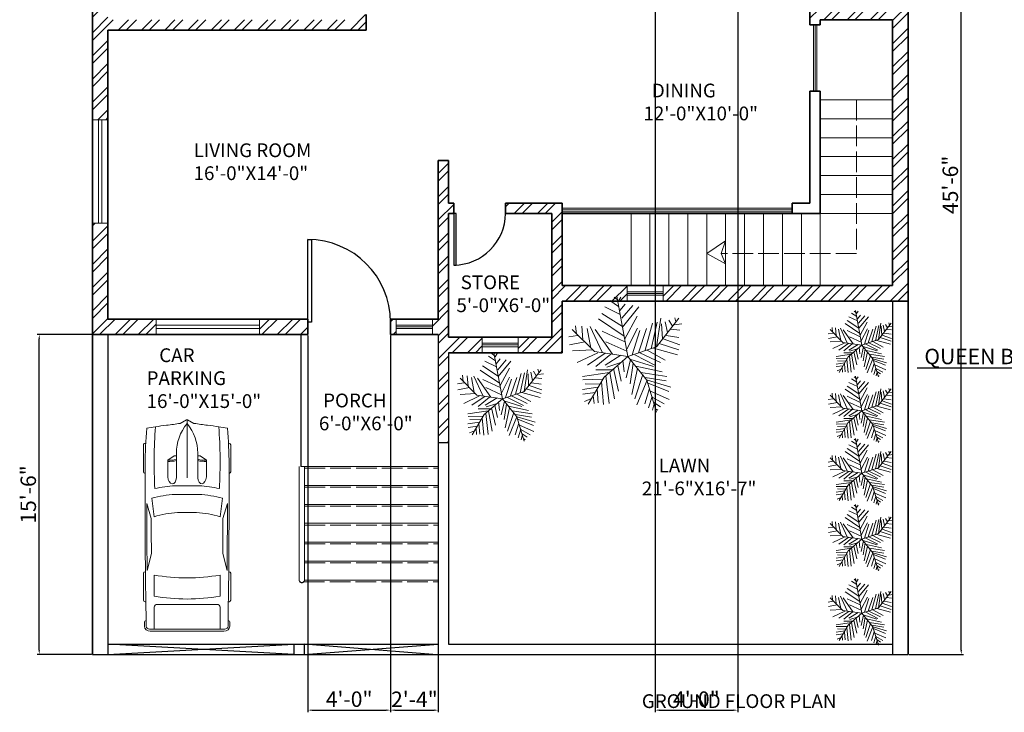
# Model space of a CAD drawing. Units: inches. Extents: x 600 to 1805, y 898 to 2057.
# Tile 2 of 5: x 600 to 1172, y 1419 to 1822. Entities that reach past the tile are written whole.
import ezdxf

# ---------------------------------------------------------------- set-up
doc = ezdxf.new("R2010")
doc.units = ezdxf.units.IN
doc.linetypes.add('ACAD_ISO02W100', pattern=[15, 12, -3])
for name, color, linetype, lineweight in [('A-ANNO-DIMS', 2, 'Continuous', 18), ('A-ANNO-PATH', 2, 'ACAD_ISO02W100', 13), ('A-ANNO-SYMB', 2, 'Continuous', 13), ('A-ANNO-TEXT', 7, 'Continuous', 25), ('A-AREA-IDEN', 7, 'Continuous', 18), ('A-DOOR', 4, 'Continuous', 25), ('A-FLOR', 7, 'Continuous', 25), ('A-FLOR-STRS', 3, 'Continuous', 20), ('A-FLOR-STRS-HIDN', 3, 'ACAD_ISO02W100', 13), ('A-WALL', 7, 'Continuous', 35), ('A-WALL-PATT', 252, 'Continuous', 13), ('C-PRKG-VEH', 8, 'Continuous', 13), ('C-SITE', 7, 'Continuous', 25), ('L-PLNT', 94, 'Continuous', 13)]:
    doc.layers.add(name, color=color, linetype=linetype, lineweight=lineweight)
doc.layers.add('A-GLAZ', color=244, linetype='Continuous', lineweight=20, true_color=0x991b1e)
doc.styles.get("Standard").update_dxf_attribs({"font": 'arial.ttf'})
doc.dimstyles.new('ISO-25', dxfattribs={"dimtxt": 9, "dimasz": 2.5, "dimexe": 1.25, "dimexo": 0.625, "dimtad": 1, "dimlunit": 3, "dimtxsty": 'Standard', "dimcen": 2.5, "dimadec": 0, "dimazin": 0, "dimtfac": 1, "dimtmove": 0, "dimatfit": 3, "dimfxl": 1, "dimarcsym": 0})

# ---------------------------------------------------------------- blocks, each defined once
blk = doc.blocks.new('*U5')
for p, q in [((0, 0), (0, 6)), ((40, 0), (40, 6))]:
    blk.add_line(p, q)
blk.add_lwpolyline([(0, 0), (0, -40), (1.75, -40), (1.75, 0)], close=True)
blk.add_arc((0, 0), 40, 270, 0)
blk = doc.blocks.new('*U2')
for p, q in [((0, 0), (0, -6)), ((40, 0), (40, -6))]:
    blk.add_line(p, q)
blk.add_lwpolyline([(0, 0), (0, 40), (1.75, 40), (1.75, 0)], close=True)
blk.add_arc((0, 0), 40, 0, 90)
blk = doc.blocks.new('*U7')
for p, q in [((21.1, 37.41), (21.1, 36.83)), ((46.55, 38.89), (22.35, 38.89)), ((47.8, 37.39), (47.8, 37.41)), ((87.99, 31.87), (74.76, 35.92)), ((134.31, 35.6), (119.29, 31.78)), ((135.45, 37.07), (135.45, 37.41)), ((136.7, 38.89), (160.9, 38.89)), ((162.15, 37.41), (162.15, 36.77)), ((70.03, 31.54), (86.41, 29.35)), ((138.42, 29.35), (157.25, 29.35)), ((164.52, 26.39), (164.52, -26.39)), ((186.47, 29.35), (167.01, 29.35)), ((186.47, -33.5), (186.47, 33.5)), ((188.4, -32.76), (188.4, 32.76)), ((29.77, 9.51), (51.68, 9.51)), ((32.12, 9.51), (32.12, 11.15)), ((32.27, 11.63), (36.13, 17.17)), ((36.13, 17.17), (50.94, 17.17)), ((58.92, -10.77), (58.92, 10.77)), ((66.55, -10.53), (66.55, 10.53)), ((186.47, -10.53), (186.47, 10.53)), ((3.27, 6.13), (0.1, 0.41)), ((82.74, 8.5), (82.74, -8.5)), ((0, 0), (51.68, 0)), ((0.1, -0.41), (3.27, -6.13)), ((29.77, -9.51), (51.68, -9.51)), ((32.12, -9.51), (32.12, -11.15)), ((32.27, -11.63), (36.13, -17.17)), ((36.13, -17.17), (50.94, -17.17)), ((86.41, -29.35), (70.03, -31.54)), ((87.99, -31.87), (74.76, -35.92)), ((134.31, -35.6), (119.29, -31.78)), ((157.25, -29.35), (138.42, -29.35)), ((167.01, -29.35), (186.47, -29.35)), ((21.1, -37.41), (21.1, -36.83)), ((46.55, -38.89), (22.35, -38.89)), ((47.8, -37.39), (47.8, -37.41)), ((135.45, -37.07), (135.45, -37.41)), ((136.7, -38.89), (160.9, -38.89)), ((162.15, -37.41), (162.15, -36.77))]:
    blk.add_line(p, q)
for centre, major_axis, ratio, start_param, end_param in [((266.03, -27.52), (0, 313.31), 0.842304, 1.367076, 1.39176), ((41.19, -490.86), (0, 528.23), 0.842304, 0.00281, 0.075598), ((22.35, 37.41), (0, -1.48), 0.842304, 3.141593, 4.712389), ((64.48, -10555.62), (0, 10593.03), 0.842304, -0.013397, 0.002797), ((46.55, 37.41), (0, 1.48), 0.842304, -1.570796, 0), ((64.48, -10555.62), (0, -10591.55), 0.842304, 3.133765, 3.140441), ((136.7, 37.41), (0, -1.48), 0.842304, 3.141593, 4.712389), ((160.9, 37.41), (0, 1.48), 0.842304, -1.570796, 0), ((180.63, 35.84), (0, 2.22), 0.842304, -0.013017, 1.249894), ((64.48, -10556.36), (0, 10595.31), 0.842304, -0.013397, -0.013017), ((183.98, 33.5), (0, -2.96), 0.842304, 1.570796, 3.128196), ((183.98, 32.76), (0, -5.25), 0.842304, 1.570796, 3.128196), ((259.18, -27.52), (0, -305.3), 0.842304, 4.528606, 4.561838), ((37.47, -593.96), (0, -623.33), 0.842304, 3.096046, 3.200911), ((134.4, 5.39), (0, -89.78), 0.842304, 4.449482, 4.652344), ((135.29, 5.39), (0, 81.77), 0.842304, 1.245306, 1.50788), ((149.6, 2.8), (0, -79.58), 0.842304, 4.372215, 4.640744), ((95.79, -3666.35), (0, -3698.24), 0.842304, 3.134049, 3.144098), ((17.08, 0), (0, 147.02), 0.842304, 4.511394, 4.913384), ((35.91, 0), (0, 147.02), 0.842304, 4.511394, 4.913384), ((167.01, 26.39), (0, 2.96), 0.842304, 0, 1.570796), ((-204.49, 52.4), (0, -250.96), 0.842304, 1.385369, 1.434372), ((29.77, -46.66), (0, 56.17), 0.842304, 0, 0.590319), ((32.75, 11.15), (0, 0.74), 0.842304, 0.879714, 1.570796), ((13.04, 17.01), (0, 27.42), 0.842304, 4.435146, 4.718221), ((14.2, 17.01), (0, 27.42), 0.842304, 4.435146, 4.718221), ((50.79, 13.34), (6.34, -0.36), 0.603834, -1.395552, 1.581315), ((0.62, 0), (0, -0.74), 0.842304, 4.131459, 5.293319), ((-204.49, -52.4), (0, 250.96), 0.842304, -1.434372, -1.385369), ((29.77, 46.66), (0, 56.17), 0.842304, 2.551274, 3.141593), ((149.6, -2.8), (0, -79.58), 0.842304, -1.499151, -1.230623), ((32.75, -11.15), (0, -0.74), 0.842304, 4.712389, 5.403472), ((13.04, -17.01), (0, -27.42), 0.842304, 1.564964, 1.848039), ((14.2, -17.01), (0, -27.42), 0.842304, 1.564964, 1.848039), ((134.4, -5.39), (0, -89.78), 0.842304, -1.510751, -1.307889), ((135.29, -5.39), (0, -81.77), 0.842304, -1.50788, -1.245306), ((259.18, 27.52), (0, 305.3), 0.842304, 1.721348, 1.754579), ((266.03, 27.52), (0, 313.31), 0.842304, 1.749832, 1.774517), ((37.47, 593.96), (0, -623.33), 0.842304, -0.059319, 0.045547), ((95.79, 3666.35), (0, -3698.24), 0.842304, -0.002505, 0.007544), ((167.01, -26.39), (0, -2.96), 0.842304, 4.712389, 6.283185), ((183.98, -33.5), (0, 2.96), 0.842304, 3.15499, 4.712389), ((183.98, -32.76), (0, -5.25), 0.842304, 0.013397, 1.570796), ((41.19, 490.86), (0, -528.23), 0.842304, -0.075598, -0.00281), ((22.35, -37.41), (0, 1.48), 0.842304, 1.570796, 3.141593), ((64.48, 10555.62), (0, 10593.03), 0.842304, 3.138796, 3.15499), ((46.55, -37.41), (0, -1.48), 0.842304, 0, 1.570796), ((64.48, 10555.62), (0, -10591.55), 0.842304, 0.001152, 0.007828), ((136.7, -37.41), (0, -1.48), 0.842304, -1.570796, 0), ((160.9, -37.41), (0, 1.48), 0.842304, 3.141593, 4.712389), ((180.63, -35.84), (0, -2.22), 0.842304, -1.249894, 0.013017), ((64.48, 10556.36), (0, 10595.31), 0.842304, 3.15461, 3.15499)]:
    blk.add_ellipse(centre, major_axis=major_axis, ratio=ratio, start_param=start_param, end_param=end_param)
at = {"extrusion": (0, 0, -1)}
blk.add_ellipse((50.79, -13.34), major_axis=(6.34, 0.36), ratio=0.603834, start_param=-1.395552, end_param=1.581315, dxfattribs=at)
blk = doc.blocks.new('*U12')
for p, q in [((-10.186, 53.64), (-13.084, 55.962)), ((0, 0), (-10.5, 57)), ((-9.099, 51.782), (-6.563, 55.962)), ((-7.288, 39.707), (-21.778, 46.673)), ((-8.737, 47.138), (-17.069, 52.711)), ((-7.65, 43.423), (-2.578, 49.46)), ((-5.839, 35.992), (4.667, 48.067)), ((-5.114, 27.632), (10.463, 46.673)), ((-5.114, 28.097), (-24.676, 40.636)), ((-2.941, 16.486), (8.652, 37.85)), ((-48.585, 21.131), (-49.309, 29.026)), ((-43.513, 28.561), (-42.427, 15.558)), ((-35.544, 28.097), (-24.314, 3.947)), ((-3.665, 19.273), (-27.574, 35.527)), ((16.259, 5.805), (23.142, 31.348)), ((22.055, 7.198), (27.489, 32.277)), ((27, 9), (48, 36)), ((27.127, 9.056), (31.112, 35.992)), ((31.836, 30.883), (32.561, 16.486)), ((35.096, 32.741), (37.27, 22.524)), ((38.719, 34.134), (41.979, 28.561)), ((43.791, 29.954), (51.036, 30.883)), ((44.153, 36.456), (45.239, 32.741)), ((-47.498, 19.737), (-55.83, 18.344)), ((-31.5, 4.5), (-52.5, 25.5)), ((-38.442, 26.239), (-34.819, 7.663)), ((-14.533, 2.09), (-30.834, 25.31)), ((-24.314, 23.917), (-2.941, 13.7)), ((-1.129, 6.734), (9.014, 26.704)), ((3.942, 1.625), (11.187, 24.381)), ((10.101, 3.483), (17.708, 26.239)), ((36.183, 19.737), (48.137, 17.88)), ((40.53, 25.775), (48.862, 24.846)), ((-40.615, 13.7), (-55.105, 10.913)), ((-20.691, 13.7), (-1.129, 4.876)), ((29.662, 12.307), (48.137, 6.269)), ((33.285, 16.486), (48.862, 10.913)), ((-33.37, 6.269), (-52.207, 5.34)), ((-28.299, 3.483), (-47.86, -5.805)), ((-21.416, 3.018), (-38.079, -8.128)), ((0, 0), (-31.5, 4.5)), ((-15.982, 2.09), (-30.11, -9.521)), ((0, 0), (-22.5, -19.5)), ((-6.563, 1.161), (-21.416, -8.128)), ((0, 0), (27, 9)), ((0, 0), (18, -22.5)), ((6.478, 1.625), (26.04, -8.592)), ((11.187, 3.483), (30.749, -5.805)), ((18.07, 5.805), (35.096, -3.483)), ((24.229, 7.663), (46.688, 1.625)), ((-6.563, -5.805), (-19.967, -9.985)), ((-9.461, -8.592), (-6.201, -23.453)), ((-4.752, -3.483), (-3.665, -14.629)), ((2.493, -3.019), (-1.491, -20.202)), ((1.769, -2.555), (24.229, -9.521)), ((5.029, -6.27), (2.131, -25.775)), ((7.565, -9.056), (32.198, -14.629)), ((-17.431, -15.094), (-42.789, -18.809)), ((-15.257, -12.772), (-30.11, -12.772)), ((-20.691, -18.345), (-17.793, -44.352)), ((-17.069, -15.094), (-12.721, -40.172)), ((-13.446, -11.378), (-8.737, -32.741)), ((9.014, -11.378), (3.58, -35.992)), ((14.085, -16.951), (6.478, -40.172)), ((12.274, -15.094), (36.907, -18.809)), ((-24.314, -21.596), (-42.427, -22.06)), ((-26.849, -26.24), (-40.253, -25.775)), ((-22.5, -19.5), (-37.5, -45)), ((-25.038, -23.918), (-22.865, -45.281)), ((18.07, -22.524), (8.289, -45.745)), ((16.259, -19.738), (36.183, -22.989)), ((18, -22.5), (27, -52.5)), ((18.433, -22.524), (40.53, -29.026)), ((19.157, -25.311), (38.719, -33.206)), ((-28.299, -29.026), (-42.789, -31.348)), ((-30.834, -34.135), (-42.427, -35.528)), ((-32.646, -36.921), (-31.921, -44.352)), ((-29.023, -30.884), (-27.936, -43.887)), ((20.244, -30.419), (15.897, -44.816)), ((21.331, -32.741), (39.081, -40.636)), ((-34.457, -39.708), (-40.978, -42.494)), ((22.78, -37.85), (19.519, -48.532)), ((22.78, -38.314), (34.372, -44.816)), ((24.591, -45.745), (23.142, -50.854)), ((24.591, -43.423), (30.749, -47.603)), ((26.764, -49.925), (28.213, -50.854))]:
    blk.add_line(p, q)
blk = doc.blocks.new('WIN-60x9')
for p, q in [((60, 5.5), (0, 5.5)), ((60, 3.5), (0, 3.5))]:
    blk.add_line(p, q)
blk.add_lwpolyline([(60, 0), (60, 9), (0, 9), (0, 0)], close=True)
blk = doc.blocks.new('VENT-21x9')
for p, q in [((0, 5.5), (21, 5.5)), ((0, 4.5), (21, 4.5)), ((0, 3.5), (21, 3.5))]:
    blk.add_line(p, q)
blk.add_lwpolyline([(21, 9), (21, 0), (0, 0), (0, 9)], close=True)
blk = doc.blocks.new('*D26')
at = {"layer": 'A-ANNO-DIMS', "color": 0, "lineweight": -2, "transparency": 16777216}
for p, q in [((1257.94, 1608), (1257.94, 1620.63)), ((1337.94, 1608), (1337.94, 1620.63)), ((1257.94, 1619.38), (1121.8, 1619.38)), ((1335.44, 1619.38), (1260.44, 1619.38))]:
    blk.add_line(p, q, dxfattribs=at)
at = {"layer": 'A-ANNO-DIMS', "color": 0, "transparency": 16777216}
for points in [[(1260.44, 1619.79), (1260.44, 1618.96), (1257.94, 1619.38)], [(1335.44, 1619.79), (1335.44, 1618.96), (1337.94, 1619.38)]]:
    blk.add_solid(points, dxfattribs=at)
at = {"layer": 'Defpoints', "color": 0, "transparency": 16777216}
for p in [(1257.94, 1619.38), (1257.94, 1607.38), (1337.94, 1607.38)]:
    blk.add_point(p, dxfattribs=at)
at = {"layer": 'A-ANNO-DIMS', "color": 0, "transparency": 16777216, "insert": (1188.62, 1624.93), "char_height": 9, "attachment_point": 5}
blk.add_mtext('QUEEN BED 6\'-8" TYP.', dxfattribs=at)
blk = doc.blocks.new('*D32')
at = {"layer": 'A-ANNO-DIMS', "color": 0, "lineweight": -2, "transparency": 16777216}
for p, q in [((1117.01, 1998.86), (1148.59, 1998.86)), ((1147.34, 1455.36), (1147.34, 1996.36)), ((1117.01, 1452.86), (1148.59, 1452.86))]:
    blk.add_line(p, q, dxfattribs=at)
at = {"layer": 'A-ANNO-DIMS', "color": 0, "transparency": 16777216}
for points in [[(1146.92, 1996.36), (1147.75, 1996.36), (1147.34, 1998.86)], [(1146.92, 1455.36), (1147.75, 1455.36), (1147.34, 1452.86)]]:
    blk.add_solid(points, dxfattribs=at)
at = {"layer": 'Defpoints', "color": 0, "transparency": 16777216}
for p in [(1116.39, 1998.86), (1147.34, 1998.86), (1116.39, 1452.86)]:
    blk.add_point(p, dxfattribs=at)
at = {"layer": 'A-ANNO-DIMS', "color": 0, "transparency": 16777216, "insert": (1142.12, 1725.86), "char_height": 9, "attachment_point": 5, "rotation": 90}
blk.add_mtext('45\'-6"', dxfattribs=at)
blk = doc.blocks.new('*D33')
at = {"layer": 'A-ANNO-DIMS', "color": 0, "lineweight": -2, "transparency": 16777216}
for p, q in [((641.76, 1638.86), (610.19, 1638.86)), ((611.44, 1455.36), (611.44, 1636.36)), ((641.76, 1452.86), (610.19, 1452.86))]:
    blk.add_line(p, q, dxfattribs=at)
at = {"layer": 'A-ANNO-DIMS', "color": 0, "transparency": 16777216}
for points in [[(611.02, 1636.36), (611.85, 1636.36), (611.44, 1638.86)], [(611.02, 1455.36), (611.85, 1455.36), (611.44, 1452.86)]]:
    blk.add_solid(points, dxfattribs=at)
at = {"layer": 'Defpoints', "color": 0, "transparency": 16777216}
for p in [(611.44, 1638.86), (642.39, 1638.86), (642.39, 1452.86)]:
    blk.add_point(p, dxfattribs=at)
at = {"layer": 'A-ANNO-DIMS', "color": 0, "transparency": 16777216, "insert": (606.22, 1545.86), "char_height": 9, "attachment_point": 5, "rotation": 90}
blk.add_mtext('15\'-6"', dxfattribs=at)
blk = doc.blocks.new('*D34')
at = {"layer": 'A-ANNO-DIMS', "color": 0, "lineweight": -2, "transparency": 16777216}
for p, q in [((815.57, 1638.23), (815.57, 1419.24)), ((843.39, 1638.23), (843.39, 1419.24)), ((818.07, 1420.49), (840.89, 1420.49))]:
    blk.add_line(p, q, dxfattribs=at)
at = {"layer": 'A-ANNO-DIMS', "color": 0, "transparency": 16777216}
for points in [[(818.07, 1420.9), (818.07, 1420.07), (815.57, 1420.49)], [(840.89, 1420.9), (840.89, 1420.07), (843.39, 1420.49)]]:
    blk.add_solid(points, dxfattribs=at)
at = {"layer": 'Defpoints', "color": 0, "transparency": 16777216}
for p in [(815.57, 1638.86), (843.39, 1638.86), (843.39, 1420.49)]:
    blk.add_point(p, dxfattribs=at)
at = {"layer": 'A-ANNO-DIMS', "color": 0, "transparency": 16777216, "insert": (829.48, 1425.63), "char_height": 9, "attachment_point": 5}
blk.add_mtext('2\'-4"', dxfattribs=at)
blk = doc.blocks.new('*D35')
at = {"layer": 'A-ANNO-DIMS', "color": 0, "lineweight": -2, "transparency": 16777216}
for p, q in [((767.57, 1638.23), (767.57, 1419.24)), ((815.57, 1638.23), (815.57, 1419.24)), ((770.07, 1420.49), (813.07, 1420.49))]:
    blk.add_line(p, q, dxfattribs=at)
at = {"layer": 'A-ANNO-DIMS', "color": 0, "transparency": 16777216}
for points in [[(770.07, 1420.9), (770.07, 1420.07), (767.57, 1420.49)], [(813.07, 1420.9), (813.07, 1420.07), (815.57, 1420.49)]]:
    blk.add_solid(points, dxfattribs=at)
at = {"layer": 'Defpoints', "color": 0, "transparency": 16777216}
for p in [(767.57, 1638.86), (815.57, 1638.86), (815.57, 1420.49)]:
    blk.add_point(p, dxfattribs=at)
at = {"layer": 'A-ANNO-DIMS', "color": 0, "transparency": 16777216, "insert": (791.57, 1425.71), "char_height": 9, "attachment_point": 5}
blk.add_mtext('4\'-0"', dxfattribs=at)
blk = doc.blocks.new('*D57')
at = {"layer": 'A-ANNO-DIMS', "color": 0, "lineweight": -2, "transparency": 16777216}
for p, q in [((969.39, 1863.23), (969.39, 1419.24)), ((1017.39, 1863.23), (1017.39, 1419.24)), ((971.89, 1420.49), (1014.89, 1420.49))]:
    blk.add_line(p, q, dxfattribs=at)
at = {"layer": 'A-ANNO-DIMS', "color": 0, "transparency": 16777216}
for points in [[(971.89, 1420.9), (971.89, 1420.07), (969.39, 1420.49)], [(1014.89, 1420.9), (1014.89, 1420.07), (1017.39, 1420.49)]]:
    blk.add_solid(points, dxfattribs=at)
at = {"layer": 'Defpoints', "color": 0, "transparency": 16777216}
for p in [(969.39, 1863.86), (1017.39, 1863.86), (1017.39, 1420.49)]:
    blk.add_point(p, dxfattribs=at)
at = {"layer": 'A-ANNO-DIMS', "color": 0, "transparency": 16777216, "insert": (993.39, 1425.71), "char_height": 9, "attachment_point": 5}
blk.add_mtext('4\'-0"', dxfattribs=at)

msp = doc.modelspace()

# ---------------------------------------------------------------- hatches: boundary and pattern name
at = {"layer": 'A-WALL-PATT'}
h = msp.add_hatch(dxfattribs=at)
h.set_pattern_fill('ANSI32', color=256)
h.paths.add_polyline_path([(651.387, 1875.859), (642.387, 1875.859), (642.387, 1763.631), (651.387, 1763.631), (651.387, 1815.859), (801.387, 1815.859), (801.387, 1824.859), (795.987, 1824.859), (795.387, 1824.859), (795.387, 1821.859), (651.387, 1821.859)])
h.paths.add_polyline_path([(795.387, 1989.859), (795.387, 1860.859), (801.387, 1860.859), (801.387, 1887.859), (804.387, 1887.859), (804.387, 1892.359), (804.387, 1893.859), (801.387, 1893.859), (801.387, 1989.859), (807.224, 1989.859), (807.224, 1998.859), (753.387, 1998.859), (753.387, 1989.859)])
h.paths.add_polyline_path([(693.387, 1989.859), (693.387, 1998.859), (642.387, 1998.859), (642.387, 1935.859), (651.387, 1935.859), (651.387, 1989.859)])
h.paths.add_polyline_path([(828.224, 1998.859), (828.224, 1989.859), (861.387, 1989.859), (861.387, 1893.859), (834.387, 1893.859), (834.387, 1887.859), (861.387, 1887.859), (894.387, 1887.859), (894.387, 1892.359), (894.387, 1893.859), (867.387, 1893.859), (867.387, 1989.859), (894.316, 1989.859), (894.316, 1998.859)])
h = msp.add_hatch(dxfattribs=at)
h.set_pattern_fill('ANSI32', color=256)
h.paths.add_polyline_path([(933.387, 1989.859), (963.387, 1989.859), (963.387, 1998.859), (915.316, 1998.859), (915.316, 1989.859), (927.387, 1989.859), (927.387, 1893.859), (924.387, 1893.859), (924.387, 1892.359), (924.387, 1887.859), (927.387, 1887.859), (927.387, 1863.859), (969.387, 1863.859), (969.387, 1869.859), (933.387, 1869.859)])
h.paths.add_polyline_path([(1059.387, 1998.859), (1023.387, 1998.859), (1023.387, 1989.859), (1053.387, 1989.859), (1053.387, 1869.859), (1017.387, 1869.859), (1017.387, 1863.859), (1062.387, 1863.859), (1062.387, 1867.459), (1062.387, 1869.859), (1059.387, 1869.859)], flags=17)
h.paths.add_polyline_path([(1116.387, 1998.859), (1107.387, 1998.859), (1107.387, 1869.859), (1086.387, 1869.859), (1086.387, 1863.859), (1107.387, 1863.859), (1107.387, 1827.859), (1059.387, 1827.859), (1059.387, 1818.859), (1065.387, 1818.859), (1065.387, 1821.859), (1107.387, 1821.859), (1107.387, 1667.256), (974.103, 1667.256), (974.103, 1658.256), (1116.387, 1658.256)])
h.paths.add_polyline_path([(953.103, 1667.256), (915.387, 1667.256), (915.387, 1715.256), (882.387, 1715.256), (882.387, 1709.256), (909.387, 1709.256), (909.387, 1637.256), (889.887, 1637.256), (889.887, 1628.256), (915.387, 1628.256), (915.387, 1658.256), (953.103, 1658.256)])
h.paths.add_polyline_path([(868.887, 1637.256), (849.387, 1637.256), (849.387, 1709.256), (852.387, 1709.256), (852.387, 1713.756), (852.387, 1715.256), (849.387, 1715.256), (849.387, 1740.017), (843.387, 1740.017), (843.387, 1647.859), (839.976, 1647.859), (839.976, 1638.859), (843.387, 1638.859), (843.387, 1576.163), (849.387, 1576.163), (849.387, 1628.256), (868.887, 1628.256)])
h.paths.add_polyline_path([(767.566, 1646.059), (767.566, 1647.859), (739.476, 1647.859), (739.476, 1638.859), (767.566, 1638.859)])
h = msp.add_hatch(dxfattribs=at)
h.set_pattern_fill('ANSI32', color=256)
h.paths.add_polyline_path([(679.476, 1647.859), (651.387, 1647.859), (651.387, 1703.631), (642.387, 1703.631), (642.387, 1638.859), (679.476, 1638.859)])
h.paths.add_polyline_path([(818.976, 1647.859), (815.566, 1647.859), (815.566, 1638.859), (818.976, 1638.859)])

# ---------------------------------------------------------------- linework, layer by layer
at = {"layer": 'A-ANNO-PATH'}
for p, q in [((1086.387, 1775.256), (1086.387, 1685.977)), ((1086.387, 1685.977), (1007.718, 1685.977))]:
    msp.add_line(p, q, dxfattribs=at)
at = {"layer": 'A-ANNO-SYMB'}
for p, q in [((999.387, 1685.977), (1010.387, 1693.236)), ((1010.387, 1693.236), (1007.718, 1685.977)), ((1010.387, 1679.972), (999.387, 1685.977)), ((1007.718, 1685.977), (1010.387, 1679.972))]:
    msp.add_line(p, q, dxfattribs=at)
at = {"layer": 'A-DOOR'}
for p, q in [((651.387, 1452.859), (759.445, 1458.859)), ((759.445, 1452.859), (651.387, 1458.859)), ((759.445, 1458.859), (759.445, 1452.859)), ((765.445, 1458.859), (765.445, 1452.859)), ((765.445, 1452.859), (843.387, 1458.859)), ((840.239, 1452.859), (765.445, 1458.859))]:
    msp.add_line(p, q, dxfattribs=at)
at = {"layer": 'A-FLOR'}
msp.add_line((763.566, 1638.859), (763.566, 1562.113), dxfattribs=at)
at = {"layer": 'A-FLOR-STRS'}
for p, q in [((1065.387, 1775.256), (1107.387, 1775.256)), ((1065.387, 1764.256), (1107.387, 1764.256)), ((1065.387, 1753.256), (1107.387, 1753.256)), ((1065.387, 1742.256), (1107.387, 1742.256)), ((1065.387, 1731.256), (1107.387, 1731.256)), ((1065.387, 1720.256), (1107.387, 1720.256)), ((955.387, 1709.256), (955.387, 1667.256)), ((966.387, 1709.256), (966.387, 1667.256)), ((977.387, 1709.256), (977.387, 1667.256)), ((988.387, 1709.256), (988.387, 1667.256)), ((999.387, 1709.256), (999.387, 1667.256)), ((1010.387, 1709.256), (1010.387, 1667.256)), ((1021.387, 1709.256), (1021.387, 1667.256)), ((1032.387, 1709.256), (1032.387, 1667.256)), ((1043.387, 1709.256), (1043.387, 1667.256)), ((1054.387, 1709.256), (1054.387, 1667.256)), ((1065.387, 1709.256), (1065.387, 1667.256)), ((1065.387, 1709.256), (1107.387, 1709.256)), ((762.566, 1562.113), (762.566, 1496.113)), ((763.566, 1562.113), (843.387, 1562.113)), ((765.566, 1562.113), (765.566, 1496.113)), ((765.566, 1551.113), (843.387, 1551.113)), ((765.566, 1540.113), (843.387, 1540.113)), ((765.566, 1529.113), (843.387, 1529.113)), ((765.566, 1518.113), (843.387, 1518.113)), ((765.566, 1507.113), (843.387, 1507.113)), ((765.566, 1496.113), (843.387, 1496.113))]:
    msp.add_line(p, q, dxfattribs=at)
for centre, radius, start, end in [((764.066, 1495.962), 1.508, 174.26491, 5.73509), ((764.066, 1496.149), 1.501, 182.13798, 357.86202)]:
    msp.add_arc(centre, radius, start, end, dxfattribs=at)
at = {"layer": 'A-FLOR-STRS-HIDN'}
for p, q in [((765.566, 1561.113), (843.387, 1561.113)), ((765.566, 1550.113), (843.387, 1550.113)), ((765.566, 1539.113), (843.387, 1539.113)), ((765.566, 1528.113), (843.387, 1528.113)), ((765.566, 1517.113), (843.387, 1517.113)), ((765.566, 1506.113), (843.387, 1506.113)), ((765.311, 1495.113), (843.387, 1495.113))]:
    msp.add_line(p, q, dxfattribs=at)
at = {"layer": 'A-GLAZ'}
for p, q in [((1061.387, 1818.859), (1061.387, 1780.295)), ((1062.387, 1818.859), (1062.387, 1780.295)), ((1063.387, 1818.859), (1063.387, 1780.295)), ((1048.968, 1712.256), (915.387, 1712.256)), ((1048.968, 1711.256), (915.387, 1711.256)), ((1048.968, 1710.256), (915.387, 1710.256))]:
    msp.add_line(p, q, dxfattribs=at)
at = {"layer": 'A-WALL'}
for p, q in [((642.387, 1998.859), (642.387, 1452.859)), ((1116.387, 1998.859), (1116.387, 1452.859)), ((1059.387, 1827.859), (1059.387, 1818.859)), ((801.387, 1824.859), (801.387, 1815.859)), ((1065.387, 1821.859), (1107.387, 1821.859)), ((1065.387, 1821.859), (1065.387, 1818.859)), ((1107.387, 1821.859), (1107.387, 1667.256)), ((651.387, 1815.859), (801.387, 1815.859)), ((651.387, 1815.859), (651.387, 1647.859)), ((1065.387, 1818.859), (1059.387, 1818.859)), ((1059.387, 1780.295), (1059.387, 1715.256)), ((1065.387, 1780.295), (1059.387, 1780.295)), ((1065.387, 1780.295), (1065.387, 1709.256)), ((843.387, 1740.017), (843.387, 1647.859)), ((843.387, 1740.017), (849.387, 1740.017)), ((849.387, 1740.017), (849.387, 1715.256)), ((849.387, 1715.256), (852.387, 1715.256)), ((852.387, 1715.256), (852.387, 1709.256)), ((882.387, 1715.256), (882.387, 1709.256)), ((882.387, 1715.256), (915.387, 1715.256)), ((915.387, 1715.256), (915.387, 1667.256)), ((1048.968, 1709.256), (1048.968, 1715.256)), ((1048.968, 1715.256), (1059.387, 1715.256)), ((849.387, 1709.256), (852.387, 1709.256)), ((849.387, 1709.256), (849.387, 1637.256)), ((882.387, 1709.256), (909.387, 1709.256)), ((909.387, 1709.256), (909.387, 1637.256)), ((915.387, 1709.256), (1065.387, 1709.256)), ((915.387, 1667.256), (1107.387, 1667.256)), ((915.387, 1658.256), (1116.387, 1658.256)), ((915.387, 1658.256), (915.387, 1628.256)), ((651.387, 1647.859), (767.566, 1647.859)), ((767.566, 1638.859), (767.566, 1647.859)), ((815.566, 1638.859), (815.566, 1647.859)), ((815.566, 1647.859), (843.387, 1647.859)), ((642.387, 1638.859), (767.566, 1638.859)), ((815.566, 1638.859), (843.387, 1638.859)), ((849.387, 1637.256), (909.387, 1637.256)), ((849.387, 1628.256), (915.387, 1628.256))]:
    msp.add_line(p, q, dxfattribs=at)
at = {"layer": 'C-SITE'}
for p, q in [((1107.387, 1658.256), (1107.387, 1452.859)), ((651.387, 1638.859), (651.387, 1452.859)), ((843.387, 1638.859), (843.387, 1452.859)), ((849.387, 1628.256), (849.387, 1458.859)), ((843.387, 1576.163), (849.387, 1576.163)), ((651.387, 1458.859), (843.387, 1458.859)), ((849.387, 1458.859), (1107.387, 1458.859)), ((642.387, 1452.859), (1116.387, 1452.859))]:
    msp.add_line(p, q, dxfattribs=at)

# ---------------------------------------------------------------- block references
at = {"layer": 'A-DOOR'}
for name, p, xscale, yscale, zscale in [('*U5', (852.387, 1709.256), 0.75, 0.75, 0.75), ('*U2', (767.566, 1646.059), 1.2, 1.2, 1.2)]:
    msp.add_blockref(name, p, dxfattribs=dict(at, xscale=xscale, yscale=yscale, zscale=zscale))
at = {"layer": 'A-GLAZ', "rotation": 90.00000000000088}
msp.add_blockref('WIN-60x9', (651.386, 1703.631), dxfattribs=at)
at = {"layer": 'A-GLAZ'}
for name, p in [('VENT-21x9', (953.103, 1658.256)), ('WIN-60x9', (679.477, 1638.859)), ('VENT-21x9', (818.976, 1638.859)), ('VENT-21x9', (868.886, 1628.256))]:
    msp.add_blockref(name, p, dxfattribs=at)
at = {"layer": 'C-PRKG-VEH', "xscale": 0.6525613319036914, "yscale": 0.6525613319036914, "zscale": 0.6525613319036914, "rotation": 270}
msp.add_blockref('*U7', (697.38, 1589.331), dxfattribs=at)
at = {"layer": 'L-PLNT'}
for p, xscale, yscale, zscale in [((953.573, 1626.113), 0.6159335180603465, 0.6159335180603465, 0.6159335180603465), ((1089.637, 1632.709), 0.3529457909039284, 0.3529457909039284, 0.3529457909039284), ((880.631, 1601.539), 0.4686933922233406, 0.4686933922233406, 0.4686933922233406), ((1089.637, 1594.527), 0.3529457909039284, 0.3529457909039284, 0.3529457909039284), ((1089.637, 1558.211), 0.3529457909039284, 0.3529457909039284, 0.3529457909039284), ((1089.637, 1519.922), 0.3529457909039284, 0.3529457909039284, 0.3529457909039284), ((1089.637, 1476.807), 0.3529457909039284, 0.3529457909039284, 0.3529457909039284)]:
    msp.add_blockref('*U12', p, dxfattribs=dict(at, xscale=xscale, yscale=yscale, zscale=zscale))

# ---------------------------------------------------------------- texts
at = {"layer": 'A-ANNO-TEXT', "insert": (961.673, 1429.724), "char_height": 8, "attachment_point": 1}
msp.add_mtext_dynamic_manual_height_columns('GROUND FLOOR PLAN', width=130.03371, gutter_width=12.5, heights=[0], dxfattribs=at)
at = {"layer": 'A-AREA-IDEN', "char_height": 8, "attachment_point": 1}
for s, width, insert in [('  DINING\\P12\'-0"X10\'-0"', 63.68907, (962.612, 1784.687)), ('LIVING ROOM\\P16\'-0"X14\'-0"', 75.22987, (701.164, 1749.954)), (' STORE\\P5\'-0"X6\'-0"', 53.01558, (853.936, 1673.21)), ('   CAR          PARKING\\P16\'-0"X15\'-0"', 63.80455, (673.853, 1630.81)), (' PORCH\\P6\'-0"X6\'-0"', 52.39171, (774.002, 1604.502)), ('    LAWN\\P21\'-6"X16\'-7"', 66.2991, (961.673, 1566.719))]:
    msp.add_mtext_dynamic_manual_height_columns(s, width=width, gutter_width=12.5, heights=[0], dxfattribs=dict(at, insert=insert))

# ---------------------------------------------------------------- dimensions: what is measured, and where the dimension line sits
at = {"layer": 'A-ANNO-DIMS'}
for base, p1, p2, picture, middle in [((1147.337, 1998.859), (1116.387, 1452.859), (1116.387, 1998.859), '*D32', (1142.116, 1725.859)), ((611.437, 1638.859), (642.387, 1452.859), (642.387, 1638.859), '*D33', (606.216, 1545.859))]:
    dim = msp.add_linear_dim(base=base, p1=p1, p2=p2, angle=90, dimstyle='ISO-25', override={"dimdec": 1, "dimlfac": 1, "dimrnd": 0, "dimzin": 1, "dimdsep": 46, "dimlunit": 4, "dimfrac": 2}, dxfattribs=at)
    dim.commit()
    dim.dimension.update_dxf_attribs({"geometry": picture, "text_midpoint": middle})
for base, p1, p2, picture, middle in [((1017.387, 1420.485), (969.387, 1863.859), (1017.387, 1863.859), '*D57', (993.387, 1425.705)), ((815.566, 1420.485), (767.566, 1638.859), (815.566, 1638.859), '*D35', (791.566, 1425.705)), ((843.387, 1420.485), (815.566, 1638.859), (843.387, 1638.859), '*D34', (829.476, 1425.629))]:
    dim = msp.add_linear_dim(base=base, p1=p1, p2=p2, dimstyle='ISO-25', override={"dimdec": 1, "dimlfac": 1, "dimrnd": 0, "dimzin": 1, "dimdsep": 46, "dimlunit": 4, "dimfrac": 2}, dxfattribs=at)
    dim.commit()
    dim.dimension.update_dxf_attribs({"geometry": picture, "text_midpoint": middle})
dim = msp.add_linear_dim(base=(1257.941, 1619.376), p1=(1337.941, 1607.376), p2=(1257.941, 1607.376), angle=180, text='QUEEN BED <> TYP.', dimstyle='ISO-25', override={"dimdec": 1, "dimlfac": 1, "dimrnd": 0, "dimzin": 1, "dimdsep": 46, "dimlunit": 4, "dimfrac": 2}, dxfattribs=at)
dim.commit()
dim.dimension.update_dxf_attribs({"geometry": '*D26', "text_midpoint": (1188.621, 1624.931)})

doc.saveas('drawing.dxf')
